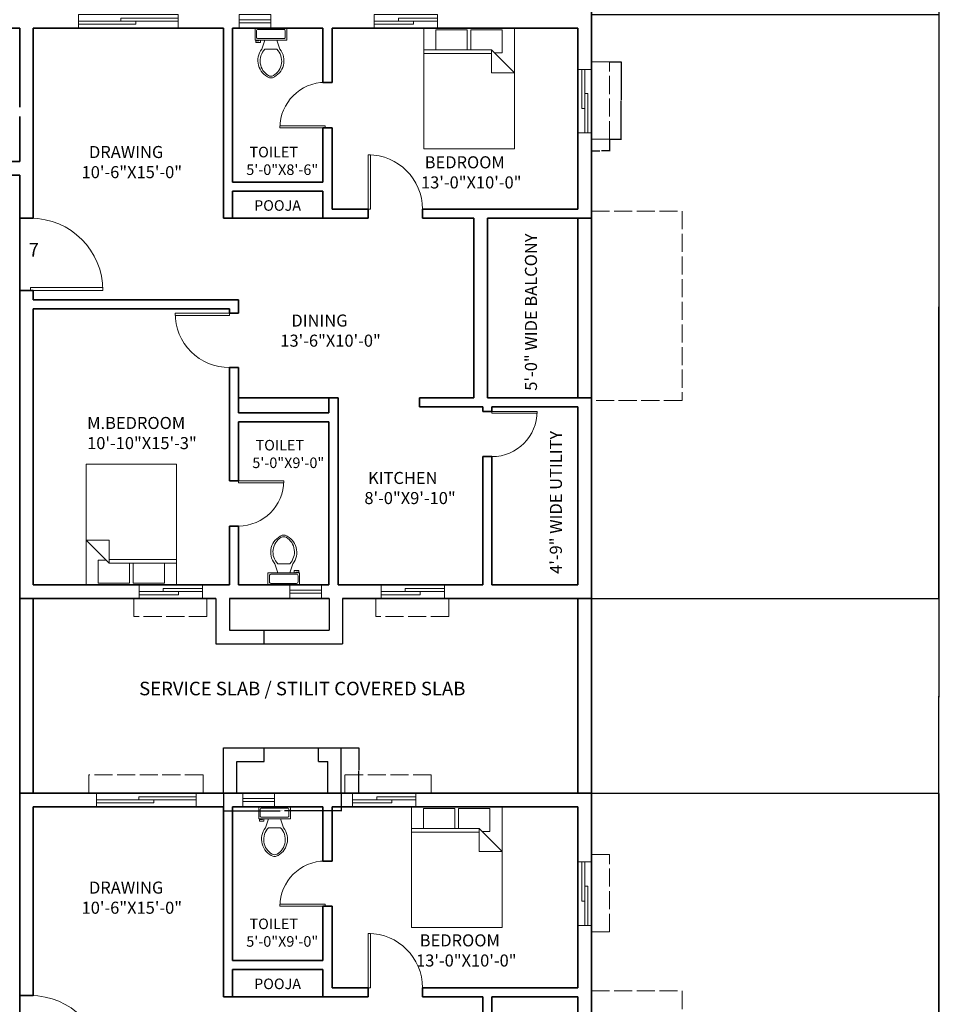
# Model space of a CAD drawing. Units: inches. Extents: x -69 to 2453, y 4803 to 7122.
# Tile 8 of 9: x 1843 to 2453, y 5759 to 6411. Entities that reach past the tile are written whole.
import ezdxf

# ---------------------------------------------------------------- set-up
doc = ezdxf.new("R2010")
doc.units = ezdxf.units.IN
doc.linetypes.add('ACAD_ISO02W100', pattern=[15, 12, -3])
for name, color, linetype, lineweight in [('A-ANNO-DIMS', 2, 'Continuous', 18), ('A-ANNO-IDEN', 2, 'Continuous', 18), ('A-AREA-IDEN', 7, 'Continuous', 18), ('A-DOOR', 3, 'Continuous', 18), ('A-FLOR-FIXT', 9, 'Continuous', 18), ('A-FLOR-OVHD', 8, 'ACAD_ISO02W100', 13), ('A-FURN', 8, 'Continuous', 18), ('A-GLAZ', 244, 'Continuous', 18), ('A-WALL', 7, 'Continuous', 35), ('A-WALL-SRVC', 7, 'Continuous', 30)]:
    doc.layers.add(name, color=color, linetype=linetype, lineweight=lineweight)
doc.styles.get("Standard").update_dxf_attribs({"font": 'arial.ttf'})
doc.dimstyles.get("Standard").update_dxf_attribs({"dimtxt": 0.18, "dimasz": 0.18, "dimexe": 0.18, "dimexo": 0.0625, "dimgap": 0.09, "dimtad": 0, "dimtih": 1, "dimtoh": 1, "dimdec": 4, "dimzin": 0, "dimdsep": 46, "dimtxsty": 'Standard', "dimcen": 0.09, "dimadec": 0, "dimazin": 0, "dimtfac": 1, "dimtdec": 4, "dimtofl": 0, "dimtmove": 0, "dimatfit": 3, "dimfxl": 1, "dimtolj": 1, "dimtzin": 0, "dimarcsym": 0})

# ---------------------------------------------------------------- blocks, each defined once
blk = doc.blocks.new('*U12')
for p, q in [((-40, 0), (-40, -6)), ((0, 0), (0, -6))]:
    blk.add_line(p, q)
blk.add_lwpolyline([(0, 0), (0, 40), (-1.75, 40), (-1.75, 0)], close=True)
blk.add_arc((0, 0), 40, 90, 180)
blk = doc.blocks.new('*U17')
for p, q in [((0, 0), (0, 6)), ((40, 0), (40, 6))]:
    blk.add_line(p, q)
blk.add_lwpolyline([(0, 0), (0, -40), (1.75, -40), (1.75, 0)], close=True)
blk.add_arc((0, 0), 40, 270, 0)
blk = doc.blocks.new('*U16')
for p, q in [((0, 0), (0, -6)), ((40, 0), (40, -6))]:
    blk.add_line(p, q)
blk.add_lwpolyline([(0, 0), (0, 40), (1.75, 40), (1.75, 0)], close=True)
blk.add_arc((0, 0), 40, 0, 90)
blk = doc.blocks.new('*U11')
for p, q in [((-40, 0), (-40, 6)), ((0, 0), (0, 6))]:
    blk.add_line(p, q)
blk.add_lwpolyline([(0, 0), (0, -40), (-1.75, -40), (-1.75, 0)], close=True)
blk.add_arc((0, 0), 40, 180, 270)
blk = doc.blocks.new('*U13')
for p, q in [((0, 0), (0, -6)), ((40, 0), (40, -6))]:
    blk.add_line(p, q)
blk.add_lwpolyline([(0, 0), (0, 40), (1.75, 40), (1.75, 0)], close=True)
blk.add_arc((0, 0), 40, 0, 90)
blk = doc.blocks.new('Bed - Queen')
for p, q in [((0, -80.00003), (0, 0)), ((0, 0), (59.99999, 0)), ((59.99999, 0), (59.99999, -80.00003)), ((7.99999, -1.2), (28.79998, -1.2)), ((7.99999, -14.4), (7.99999, -1.2)), ((28.79998, -1.2), (28.79998, -14.4)), ((31.19999, -1.2), (51.99999, -1.2)), ((31.19999, -14.4), (31.19999, -1.2)), ((51.99999, -1.2), (51.99999, -16.4)), ((0, -14.4), (44.8, -14.4)), ((44.8, -16.8), (0, -16.8)), ((59.99999, -29.6), (44.8, -14.4)), ((44.8, -14.4), (44.8, -29.6)), ((51.99999, -16.4), (46.79936, -16.4)), ((44.8, -29.6), (59.99999, -29.6)), ((59.99999, -80.00003), (0, -80.00003))]:
    blk.add_line(p, q)
blk = doc.blocks.new('*U33')
for p, q in [((9.5, -6), (9.5, -2)), ((-10, -8.5), (-8, -8.5)), ((-10, -9.5), (-10, -8.5)), ((-7, -9.5), (-10, -9.5)), ((-8, -8.5), (-8, -8)), ((-7, -8), (-7, -9.5)), ((-4, -8), (-6, -14)), ((4, -8), (6, -14)), ((4, -14), (-4, -14))]:
    blk.add_line(p, q)
blk.add_lwpolyline([(10.5, -8), (10.5, 0), (-10.5, 0), (-10.5, -8)], close=True)
for points in [[(-9.5, -2), (-9.5, -6)], [(8.5, -1), (-8.5, -1)], [(-8.5, -7), (8.5, -7)]]:
    blk.add_lwpolyline(points)
for centre, radius, start, end in [((-8.62, -1.88), 0.884, 81.8699, 188.1301), ((-8.62, -6.12), 0.884, 171.8699, 278.1301), ((8.62, -1.88), 0.884, 351.8699, 98.1301), ((8.62, -6.12), 0.884, 261.8699, 8.1301), ((3.52, -21.58), 12.17, 141.46911, 247.97143), ((4.2, -21.82), 11.33, 136.36773, 238.94682), ((-3.52, -21.58), 12.17, 292.02843, 38.53071), ((-4.2, -21.82), 11.33, 301.05301, 43.63209), ((0, -27.88), 4, 245.73182, 294.26817), ((0, -29), 4, 254.86053, 285.13947)]:
    blk.add_arc(centre, radius, start, end)
blk = doc.blocks.new('WINDOW-VENT-21IN')
for p, q in [((0, 5.5), (21, 5.5)), ((0, 3.5), (21, 3.5))]:
    blk.add_line(p, q)
blk.add_lwpolyline([(0, 9), (21, 9), (21, 0), (0, 0)], close=True)
blk = doc.blocks.new('WINDOW-SLIDING-42IN')
for p, q in [((2.5, 42), (2.5, 16)), ((4.5, 42), (4.5, 0)), ((4.5, 26), (6.5, 26)), ((6.5, 26), (6.5, 0)), ((4.5, 16), (2.5, 16))]:
    blk.add_line(p, q)
blk.add_lwpolyline([(0, 42), (9, 42), (9, 0), (0, 0)], close=True)
blk = doc.blocks.new('WINDOW-SLIDING-66IN')
for p, q in [((66, 4.5), (0, 4.5)), ((38, 2.5), (0, 2.5)), ((66, 6.5), (28, 6.5)), ((28, 4.5), (28, 6.5)), ((38, 4.5), (38, 2.5))]:
    blk.add_line(p, q)
blk.add_lwpolyline([(66, 9), (66, 0), (0, 0), (0, 9)], close=True)
blk = doc.blocks.new('SUNSHADE-48IN')
for p, q in [((0, 0), (0, 12)), ((48.4, 12), (48.4, 0)), ((48.4, 0), (0, 0))]:
    blk.add_line(p, q)
blk = doc.blocks.new('SUNSHADE-57IN')
for p, q in [((57.14, 12), (0, 12)), ((0, 12), (0, 0)), ((57.14, 0), (57.14, 12))]:
    blk.add_line(p, q)
blk = doc.blocks.new('SUNSHADE-51IN')
for p, q in [((12, 51.36), (0, 51.36)), ((12, 0), (12, 51.36)), ((0, 0), (12, 0))]:
    blk.add_line(p, q)
blk = doc.blocks.new('SUNSHADE-76IN')
for p, q in [((75.65, 12), (0, 12)), ((0, 12), (0, 0)), ((75.65, 0), (75.65, 12))]:
    blk.add_line(p, q)
blk = doc.blocks.new('SERVICE-BAY-78IN')
for p, q in [((0, 30), (78.14, 30)), ((0, 0), (0, 30)), ((27.07, 21), (27.07, 30)), ((63.07, 21), (63.07, 30)), ((78.14, 0), (78.14, 30)), ((9, 0), (9, 21)), ((9, 21), (27.07, 21)), ((63.07, 21), (69.14, 21)), ((69.14, 0), (69.14, 21))]:
    blk.add_line(p, q)
blk = doc.blocks.new('*D65')
at = {"layer": 'A-ANNO-DIMS', "color": 0, "lineweight": -2, "transparency": 16777216}
for p, q in [((2234.07, 6383.4), (2241.89, 6383.4)), ((2241.71, 6383.22), (2241.71, 6357.9)), ((2241.71, 6332.22), (2241.71, 6357.53)), ((2234.07, 6332.04), (2241.89, 6332.04))]:
    blk.add_line(p, q, dxfattribs=at)
at = {"layer": 'A-ANNO-DIMS', "color": 0, "transparency": 16777216}
for points in [[(2241.68, 6383.22), (2241.74, 6383.22), (2241.71, 6383.4)], [(2241.68, 6332.22), (2241.74, 6332.22), (2241.71, 6332.04)]]:
    blk.add_solid(points, dxfattribs=at)
at = {"layer": 'Defpoints', "color": 0, "transparency": 16777216}
for p in [(2234.01, 6383.4), (2241.71, 6383.4), (2234.01, 6332.04)]:
    blk.add_point(p, dxfattribs=at)
at = {"layer": 'A-ANNO-DIMS', "color": 0, "transparency": 16777216, "insert": (2241.71, 6357.72), "char_height": 0.18, "attachment_point": 5}
blk.add_mtext('\\A1;SUNSHADE 51 TYP.', dxfattribs=at)
blk = doc.blocks.new('*D66')
at = {"layer": 'A-ANNO-DIMS', "color": 0, "lineweight": -2, "transparency": 16777216}
for p, q in [((2222.01, 6331.97), (2222.01, 6324.15)), ((2234.01, 6331.97), (2234.01, 6324.15)), ((2222.19, 6324.33), (2227.49, 6324.33)), ((2233.83, 6324.33), (2228.53, 6324.33))]:
    blk.add_line(p, q, dxfattribs=at)
at = {"layer": 'A-ANNO-DIMS', "color": 0, "transparency": 16777216}
for points in [[(2222.19, 6324.36), (2222.19, 6324.3), (2222.01, 6324.33)], [(2233.83, 6324.36), (2233.83, 6324.3), (2234.01, 6324.33)]]:
    blk.add_solid(points, dxfattribs=at)
at = {"layer": 'Defpoints', "color": 0, "transparency": 16777216}
for p in [(2222.01, 6332.04), (2234.01, 6332.04), (2234.01, 6324.33)]:
    blk.add_point(p, dxfattribs=at)
at = {"layer": 'A-ANNO-DIMS', "color": 0, "transparency": 16777216, "insert": (2228.01, 6324.33), "char_height": 0.18, "attachment_point": 5}
blk.add_mtext('\\A1;12 TYP.', dxfattribs=at)
blk = doc.blocks.new('*D69')
at = {"layer": 'A-ANNO-DIMS', "color": 0, "lineweight": -2, "transparency": 16777216}
for p, q in [((1978.01, 5898.65), (1978.01, 5886.81)), ((2056.15, 5898.65), (2056.15, 5886.81)), ((1978.19, 5886.99), (2015.68, 5886.99)), ((2055.97, 5886.99), (2018.48, 5886.99))]:
    blk.add_line(p, q, dxfattribs=at)
at = {"layer": 'A-ANNO-DIMS', "color": 0, "transparency": 16777216}
for points in [[(1978.19, 5887.02), (1978.19, 5886.96), (1978.01, 5886.99)], [(2055.97, 5887.02), (2055.97, 5886.96), (2056.15, 5886.99)]]:
    blk.add_solid(points, dxfattribs=at)
at = {"layer": 'Defpoints', "color": 0, "transparency": 16777216}
for p in [(1978.01, 5898.72), (2056.15, 5898.72), (2056.15, 5886.99)]:
    blk.add_point(p, dxfattribs=at)
at = {"layer": 'A-ANNO-DIMS', "color": 0, "transparency": 16777216, "insert": (2017.08, 5886.99), "char_height": 0.18, "attachment_point": 5}
blk.add_mtext('\\A1;SERVICE BAY 78 TYP.', dxfattribs=at)
blk = doc.blocks.new('*D70')
at = {"layer": 'A-ANNO-DIMS', "color": 0, "lineweight": -2, "transparency": 16777216}
for p, q in [((2056.21, 5928.72), (2068.05, 5928.72)), ((2067.87, 5928.54), (2067.87, 5913.9)), ((2067.87, 5898.9), (2067.87, 5913.53)), ((2056.21, 5898.72), (2068.05, 5898.72))]:
    blk.add_line(p, q, dxfattribs=at)
at = {"layer": 'A-ANNO-DIMS', "color": 0, "transparency": 16777216}
for points in [[(2067.84, 5928.54), (2067.9, 5928.54), (2067.87, 5928.72)], [(2067.84, 5898.9), (2067.9, 5898.9), (2067.87, 5898.72)]]:
    blk.add_solid(points, dxfattribs=at)
at = {"layer": 'Defpoints', "color": 0, "transparency": 16777216}
for p in [(2056.15, 5928.72), (2067.87, 5928.72), (2056.15, 5898.72)]:
    blk.add_point(p, dxfattribs=at)
at = {"layer": 'A-ANNO-DIMS', "color": 0, "transparency": 16777216, "insert": (2067.87, 5913.72), "char_height": 0.18, "attachment_point": 5}
blk.add_mtext('\\A1;30 TYP.', dxfattribs=at)
blk = doc.blocks.new('*D90')
at = {"layer": 'A-ANNO-DIMS', "color": 0, "lineweight": -2, "transparency": 16777216}
for p, q in [((2222.07, 5898.72), (2452.44, 5898.72)), ((2452.26, 5898.54), (2452.26, 5705.4)), ((2452.26, 5511.9), (2452.26, 5705.03)), ((2222.07, 5511.72), (2452.44, 5511.72))]:
    blk.add_line(p, q, dxfattribs=at)
at = {"layer": 'A-ANNO-DIMS', "color": 0, "transparency": 16777216}
for points in [[(2452.23, 5898.54), (2452.29, 5898.54), (2452.26, 5898.72)], [(2452.23, 5511.9), (2452.29, 5511.9), (2452.26, 5511.72)]]:
    blk.add_solid(points, dxfattribs=at)
at = {"layer": 'Defpoints', "color": 0, "transparency": 16777216}
for p in [(2222.01, 5898.72), (2452.26, 5898.72), (2222.01, 5511.72)]:
    blk.add_point(p, dxfattribs=at)
at = {"layer": 'A-ANNO-DIMS', "color": 0, "transparency": 16777216, "insert": (2452.26, 5705.22), "char_height": 0.18, "attachment_point": 5}
blk.add_mtext('\\A1;387', dxfattribs=at)
blk = doc.blocks.new('*D91')
at = {"layer": 'A-ANNO-DIMS', "color": 0, "lineweight": -2, "transparency": 16777216}
for p, q in [((2222.07, 6027.72), (2452.44, 6027.72)), ((2452.26, 6027.54), (2452.26, 5963.4)), ((2452.26, 5898.9), (2452.26, 5963.03)), ((2222.07, 5898.72), (2452.44, 5898.72))]:
    blk.add_line(p, q, dxfattribs=at)
at = {"layer": 'A-ANNO-DIMS', "color": 0, "transparency": 16777216}
for points in [[(2452.23, 6027.54), (2452.29, 6027.54), (2452.26, 6027.72)], [(2452.23, 5898.9), (2452.29, 5898.9), (2452.26, 5898.72)]]:
    blk.add_solid(points, dxfattribs=at)
at = {"layer": 'Defpoints', "color": 0, "transparency": 16777216}
for p in [(2222.01, 6027.72), (2452.26, 6027.72), (2222.01, 5898.72)]:
    blk.add_point(p, dxfattribs=at)
at = {"layer": 'A-ANNO-DIMS', "color": 0, "transparency": 16777216, "insert": (2452.26, 5963.22), "char_height": 0.18, "attachment_point": 5}
blk.add_mtext('\\A1;129', dxfattribs=at)
blk = doc.blocks.new('*D92')
at = {"layer": 'A-ANNO-DIMS', "color": 0, "lineweight": -2, "transparency": 16777216}
for p, q in [((2222.07, 6414.72), (2452.44, 6414.72)), ((2452.26, 6414.54), (2452.26, 6221.4)), ((2452.26, 6027.9), (2452.26, 6221.03)), ((2222.07, 6027.72), (2452.44, 6027.72))]:
    blk.add_line(p, q, dxfattribs=at)
at = {"layer": 'A-ANNO-DIMS', "color": 0, "transparency": 16777216}
for points in [[(2452.23, 6414.54), (2452.29, 6414.54), (2452.26, 6414.72)], [(2452.23, 6027.9), (2452.29, 6027.9), (2452.26, 6027.72)]]:
    blk.add_solid(points, dxfattribs=at)
at = {"layer": 'Defpoints', "color": 0, "transparency": 16777216}
for p in [(2222.01, 6414.72), (2452.26, 6414.72), (2222.01, 6027.72)]:
    blk.add_point(p, dxfattribs=at)
at = {"layer": 'A-ANNO-DIMS', "color": 0, "transparency": 16777216, "insert": (2452.26, 6221.22), "char_height": 0.18, "attachment_point": 5}
blk.add_mtext('\\A1;387', dxfattribs=at)
blk = doc.blocks.new('*D96')
at = {"layer": 'A-ANNO-DIMS', "color": 0, "lineweight": -2, "transparency": 16777216}
for p, q in [((2044.63, 7006.72), (2452.44, 7006.72)), ((2452.26, 7006.54), (2452.26, 5962.4)), ((2452.26, 4917.9), (2452.26, 5962.03)), ((2143.12, 4917.72), (2452.44, 4917.72))]:
    blk.add_line(p, q, dxfattribs=at)
at = {"layer": 'A-ANNO-DIMS', "color": 0, "transparency": 16777216}
for points in [[(2452.23, 7006.54), (2452.29, 7006.54), (2452.26, 7006.72)], [(2452.23, 4917.9), (2452.29, 4917.9), (2452.26, 4917.72)]]:
    blk.add_solid(points, dxfattribs=at)
at = {"layer": 'Defpoints', "color": 0, "transparency": 16777216}
for p in [(2044.57, 7006.72), (2452.26, 7006.72), (2143.06, 4917.72)]:
    blk.add_point(p, dxfattribs=at)
at = {"layer": 'A-ANNO-DIMS', "color": 0, "transparency": 16777216, "insert": (2452.26, 5962.22), "char_height": 0.18, "attachment_point": 5}
blk.add_mtext('\\A1;2089', dxfattribs=at)

msp = doc.modelspace()

# ---------------------------------------------------------------- linework, layer by layer
at = {"layer": 'A-FLOR-OVHD'}
for p, q in [((2222.01, 6284.36), (2282.01, 6284.36)), ((2282.01, 6284.36), (2282.01, 6158.85)), ((2282.01, 6158.85), (2222.01, 6158.85)), ((2222.01, 5767.63), (2282.01, 5767.63)), ((2282.01, 5767.63), (2282.01, 5646.75))]:
    msp.add_line(p, q, dxfattribs=at)
at = {"layer": 'A-WALL'}
for p, q in [((2222.01, 6543.72), (2222.01, 5382.72)), ((1758.51, 6405.72), (1843.01, 6405.72)), ((1843.01, 6405.72), (1843.01, 6353.22)), ((1852.01, 6405.72), (1852.01, 6279.72)), ((1852.01, 6405.72), (1978.01, 6405.72)), ((1978.01, 6405.72), (1978.01, 6279.72)), ((1984.01, 6405.72), (1984.01, 6303.72)), ((1984.01, 6405.72), (2044.01, 6405.72)), ((2044.01, 6405.72), (2044.01, 6369.72)), ((2050.01, 6405.72), (2050.01, 6369.72)), ((2050.01, 6405.72), (2213.01, 6405.72)), ((2213.01, 6405.72), (2213.01, 6285.72)), ((2044.01, 6369.72), (2050.01, 6369.72)), ((1843.01, 6347.22), (1843.01, 6317.22)), ((2044.01, 6339.72), (2050.01, 6339.72)), ((2044.01, 6339.72), (2044.01, 6303.72)), ((2050.01, 6339.72), (2050.01, 6285.72)), ((1814.76, 6317.22), (1843.01, 6317.22)), ((1749.51, 6308.22), (1843.01, 6308.22)), ((1843.01, 6308.22), (1843.01, 5382.72)), ((1984.01, 6303.72), (2044.01, 6303.72)), ((1984.01, 6297.72), (2044.01, 6297.72)), ((1984.01, 6297.72), (1984.01, 6279.72)), ((2044.01, 6297.72), (2044.01, 6279.72)), ((2050.01, 6285.72), (2074.01, 6285.72)), ((2074.01, 6285.72), (2074.01, 6279.72)), ((2110.01, 6285.72), (2110.01, 6279.72)), ((2110.01, 6285.72), (2213.01, 6285.72)), ((1852.01, 6279.72), (1843.01, 6279.72)), ((1978.01, 6279.72), (2074.01, 6279.72)), ((2110.01, 6279.72), (2144.01, 6279.72)), ((2144.01, 6279.72), (2144.01, 6160.72)), ((2153.01, 6279.72), (2153.01, 6160.72)), ((2153.01, 6279.72), (2222.01, 6279.72)), ((2213.01, 6279.72), (2213.01, 6160.72)), ((1852.01, 6231.72), (1843.01, 6231.72)), ((1852.01, 6231.72), (1852.01, 6225.72)), ((1852.01, 6225.72), (1988.01, 6225.72)), ((1988.01, 6225.72), (1988.01, 6216.72)), ((1852.01, 6219.72), (1982.01, 6219.72)), ((1852.01, 6219.72), (1852.01, 6036.72)), ((1982.01, 6219.72), (1982.01, 6216.72)), ((1982.01, 6216.72), (1988.01, 6216.72)), ((1982.01, 6180.72), (1988.01, 6180.72)), ((1982.01, 6180.72), (1982.01, 6105.72)), ((1988.01, 6180.72), (1988.01, 6150.72)), ((1988.01, 6160.72), (2054.01, 6160.72)), ((2048.01, 6160.72), (2048.01, 6150.72)), ((2054.01, 6160.72), (2054.01, 6036.72)), ((2108.01, 6160.72), (2108.01, 6154.72)), ((2108.01, 6160.72), (2144.01, 6160.72)), ((2153.01, 6160.72), (2222.01, 6160.72)), ((2150.01, 6154.72), (2108.01, 6154.72)), ((2150.01, 6154.72), (2150.01, 6151.72)), ((2156.01, 6154.72), (2156.01, 6151.72)), ((2156.01, 6154.72), (2213.01, 6154.72)), ((2213.01, 6154.72), (2213.01, 6036.72)), ((1988.01, 6150.72), (2048.01, 6150.72)), ((2150.01, 6151.72), (2156.01, 6151.72)), ((1988.01, 6144.72), (2048.01, 6144.72)), ((1988.01, 6144.72), (1988.01, 6105.72)), ((2048.01, 6144.72), (2048.01, 6036.72)), ((2150.01, 6121.72), (2156.01, 6121.72)), ((2150.01, 6121.72), (2150.01, 6036.72)), ((2156.01, 6121.72), (2156.01, 6036.72)), ((1988.01, 6105.72), (1982.01, 6105.72)), ((1988.01, 6075.72), (1982.01, 6075.72)), ((1982.01, 6075.72), (1982.01, 6036.72)), ((1988.01, 6075.72), (1988.01, 6036.72)), ((1852.01, 6036.72), (1982.01, 6036.72)), ((1988.01, 6036.72), (2048.01, 6036.72)), ((2054.01, 6036.72), (2150.01, 6036.72)), ((2156.01, 6036.72), (2213.01, 6036.72)), ((1843.01, 6027.72), (1973.01, 6027.72)), ((1852.01, 6027.72), (1852.01, 5898.72)), ((1982.01, 6027.72), (2048.06, 6027.72)), ((2057.06, 6027.72), (2222.01, 6027.72)), ((2213.01, 6027.72), (2213.01, 5898.72)), ((1843.01, 5898.72), (2222.01, 5898.72)), ((1852.01, 5889.72), (1978.01, 5889.72)), ((1852.01, 5889.72), (1852.01, 5764.52)), ((1978.01, 5889.72), (1978.01, 5763.72)), ((1984.01, 5889.72), (1984.01, 5787.72)), ((1984.01, 5889.72), (2044.01, 5889.72)), ((2044.01, 5889.72), (2044.01, 5853.72)), ((2050.01, 5889.72), (2050.01, 5853.72)), ((2050.01, 5889.72), (2213.01, 5889.72)), ((2213.01, 5889.72), (2213.01, 5769.72)), ((2044.01, 5853.72), (2050.01, 5853.72)), ((2044.01, 5823.72), (2050.01, 5823.72)), ((2044.01, 5823.72), (2044.01, 5787.72)), ((2050.01, 5823.72), (2050.01, 5769.72)), ((1984.01, 5787.72), (2044.01, 5787.72)), ((1984.01, 5781.72), (2044.01, 5781.72)), ((1984.01, 5781.72), (1984.01, 5763.72)), ((2044.01, 5781.72), (2044.01, 5763.72)), ((2050.01, 5769.72), (2074.01, 5769.72)), ((2074.01, 5769.72), (2074.01, 5763.72)), ((2110.01, 5769.72), (2110.01, 5763.72)), ((2110.01, 5769.72), (2213.01, 5769.72)), ((1852.01, 5764.52), (1843.01, 5764.52)), ((1978.01, 5763.72), (2074.01, 5763.72)), ((2110.01, 5763.72), (2150.01, 5763.72)), ((2150.01, 5763.72), (2150.01, 5648.72)), ((2156.01, 5763.72), (2156.01, 5648.72)), ((2156.01, 5763.72), (2213.01, 5763.72)), ((2213.01, 5763.72), (2213.01, 5648.72))]:
    msp.add_line(p, q, dxfattribs=at)
at = {"layer": 'A-WALL-SRVC'}
for p, q in [((1973.01, 6027.72), (1973.01, 5997.72)), ((1982.01, 6027.72), (1982.01, 6006.72)), ((2048.06, 6027.72), (2048.06, 6006.72)), ((2057.06, 6027.72), (2057.06, 5997.72)), ((1982.01, 6006.72), (2048.06, 6006.72)), ((2004.83, 6006.72), (2004.83, 5997.72)), ((1973.01, 5997.72), (2057.06, 5997.72))]:
    msp.add_line(p, q, dxfattribs=at)

# ---------------------------------------------------------------- block references
at = {"layer": 'A-DOOR'}
for name, p, xscale, yscale, zscale, rotation in [('*U11', (2045.51, 6339.72), 0.75, 0.75, 0.75, 270.0000000000001), ('*U12', (1850.21, 6231.72), 1.199999999999977, 1.199999999999977, 1.199999999999977, 270.0000000000001), ('*U17', (1982.01, 6216.72), 0.9, 0.9, 0.9, 270), ('*U13', (2156.01, 6151.72), 0.75, 0.75, 0.75, 270.0000000000001), ('*U13', (1988.01, 6105.72), 0.75, 0.75, 0.75, 270.0000000000001), ('*U11', (2045.51, 5823.72), 0.75, 0.75, 0.75, 270.0000000000001), ('*U12', (1850.21, 5716.52), 1.199999999999977, 1.199999999999977, 1.199999999999977, 270.0000000000001)]:
    msp.add_blockref(name, p, dxfattribs=dict(at, xscale=xscale, yscale=yscale, zscale=zscale, rotation=rotation))
at = {"layer": 'A-DOOR', "xscale": 0.9, "yscale": 0.9, "zscale": 0.9}
for p in [(2074.01, 6285.72), (2074.01, 5769.72)]:
    msp.add_blockref('*U16', p, dxfattribs=at)
at = {"layer": 'A-FLOR-FIXT'}
for p in [(2009.52, 6405.72), (2011.93, 5889.72)]:
    msp.add_blockref('*U33', p, dxfattribs=at)
at = {"layer": 'A-FLOR-FIXT', "rotation": 180}
msp.add_blockref('*U33', (2018.01, 6036.72), dxfattribs=at)
at = {"layer": 'A-FLOR-OVHD'}
for name, p in [('SUNSHADE-51IN', (2222.01, 6332.04)), ('SUNSHADE-48IN', (1918.74, 6015.72)), ('SUNSHADE-48IN', (2079.05, 6015.72)), ('SUNSHADE-76IN', (1888.88, 5898.72)), ('SUNSHADE-57IN', (2058.57, 5898.72)), ('SUNSHADE-51IN', (2222.01, 5806.72))]:
    msp.add_blockref(name, p, dxfattribs=at)
at = {"layer": 'A-FURN'}
for p in [(2110.87, 6405.72), (2102.71, 5889.72)]:
    msp.add_blockref('Bed - Queen', p, dxfattribs=at)
at = {"layer": 'A-FURN', "rotation": 180}
msp.add_blockref('Bed - Queen', (1947.01, 6036.72), dxfattribs=at)
at = {"layer": 'A-GLAZ'}
for name, p in [('WINDOW-SLIDING-66IN', (1882.01, 6405.72)), ('WINDOW-VENT-21IN', (1988.52, 6405.72)), ('WINDOW-SLIDING-42IN', (2213.01, 6336.37)), ('WINDOW-VENT-21IN', (2021.99, 6027.72)), ('WINDOW-SLIDING-66IN', (1893.95, 5889.72)), ('WINDOW-VENT-21IN', (1990.93, 5889.72)), ('WINDOW-SLIDING-42IN', (2213.01, 5811.06))]:
    msp.add_blockref(name, p, dxfattribs=at)
for p, rotation in [((2078.01, 6414.72), 270.0000000000009), ((1922.19, 6036.72), 269.9999999999988), ((2082.5, 6036.72), 270.0000000000009), ((2063.66, 5898.72), 269.9999999999984)]:
    msp.add_blockref('WINDOW-SLIDING-42IN', p, dxfattribs=dict(at, rotation=rotation))
at = {"layer": 'A-WALL-SRVC'}
msp.add_blockref('SERVICE-BAY-78IN', (1978.01, 5898.72), dxfattribs=at)

# ---------------------------------------------------------------- texts
at = {"layer": 'A-ANNO-IDEN', "insert": (1848.93, 6263.27), "char_height": 8, "attachment_point": 1}
msp.add_mtext_dynamic_manual_height_columns('{\\H1.125x;7} ', width=10.4994, gutter_width=12.5, heights=[0], dxfattribs=at)
at = {"layer": 'A-AREA-IDEN', "attachment_point": 1}
for s, width, insert, char_height in [('  DRAWING\\P10\'-6"X15\'-0"', 66.0939, (1884.05, 6327.59), 8), (' TOILET\\P5\'-0"X8\'-6"', 45.2002, (1993.2, 6327.06), 7), (' BEDROOM\\P13\'-0"X10\'-0"', 64.9911, (2109.01, 6320.78), 8), ('POOJA', 33.9191, (1998.36, 6291.65), 7), ('   DINING\\P13\'-6"X10\'-0"', 63.2359, (2015.77, 6215.9), 8), ('M.BEDROOM\\P10\'-10"X15\'-3"', 69.6032, (1887.72, 6148.02), 8), (' TOILET\\P5\'-0"X9\'-0"', 45.2002, (1997.2, 6132.8), 7), (' KITCHEN\\P8\'-0"X9\'-10"', 58.1282, (2071.46, 6111.59), 8), ('SERVICE SLAB / STILIT COVERED SLAB', 244.2019, (1922.18, 5972.53), 9), ('  DRAWING\\P10\'-6"X15\'-0"', 66.0939, (1884.05, 5840.09), 8), (' TOILET\\P5\'-0"X9\'-0"', 45.2002, (1993.2, 5815.57), 7), (' BEDROOM\\P13\'-0"X10\'-0"', 64.9911, (2105.73, 5805.11), 8), ('POOJA', 33.9191, (1998.36, 5775.79), 7)]:
    msp.add_mtext_dynamic_manual_height_columns(s, width=width, gutter_width=12.5, heights=[0], dxfattribs=dict(at, insert=insert, char_height=char_height))
at = {"layer": 'A-AREA-IDEN', "char_height": 8, "attachment_point": 1, "rotation": 90}
for s, width, insert in [('5\'-0" WIDE BALCONY', 114.3745, (2177.88, 6165.4)), ('4\'-9" WIDE UTILITY', 99.5525, (2194.4, 6044.01))]:
    msp.add_mtext_dynamic_manual_height_columns(s, width=width, gutter_width=12.5, heights=[0], dxfattribs=dict(at, insert=insert))

# ---------------------------------------------------------------- dimensions: what is measured, and where the dimension line sits
at = {"layer": 'A-ANNO-DIMS'}
for base, p1, p2, picture, middle in [((2452.26, 7006.72), (2143.06, 4917.72), (2044.57, 7006.72), '*D96', (2452.26, 5962.22)), ((2452.26, 6414.72), (2222.01, 6027.72), (2222.01, 6414.72), '*D92', (2452.26, 6221.22)), ((2452.26, 6027.72), (2222.01, 5898.72), (2222.01, 6027.72), '*D91', (2452.26, 5963.22)), ((2452.26, 5898.72), (2222.01, 5511.72), (2222.01, 5898.72), '*D90', (2452.26, 5705.22))]:
    dim = msp.add_linear_dim(base=base, p1=p1, p2=p2, angle=90, dimstyle='Standard', override={"dimdec": 0, "dimlfac": 1, "dimrnd": 0, "dimzin": 0, "dimdsep": 46, "dimlunit": 2}, dxfattribs=at)
    dim.commit()
    dim.dimension.update_dxf_attribs({"geometry": picture, "text_midpoint": middle})
for base, p1, p2, text, picture, middle in [((2241.71, 6383.4), (2234.01, 6332.04), (2234.01, 6383.4), 'SUNSHADE <> TYP.', '*D65', (2241.71, 6357.72)), ((2067.87, 5928.72), (2056.15, 5898.72), (2056.15, 5928.72), '<> TYP.', '*D70', (2067.87, 5913.72))]:
    dim = msp.add_linear_dim(base=base, p1=p1, p2=p2, angle=90, text=text, dimstyle='Standard', override={"dimdec": 0, "dimlfac": 1, "dimrnd": 0, "dimzin": 0, "dimdsep": 46, "dimlunit": 2}, dxfattribs=at)
    dim.commit()
    dim.dimension.update_dxf_attribs({"geometry": picture, "text_midpoint": middle})
for base, p1, p2, text, picture, middle in [((2234.01, 6324.33), (2222.01, 6332.04), (2234.01, 6332.04), '<> TYP.', '*D66', (2228.01, 6324.33)), ((2056.15, 5886.99), (1978.01, 5898.72), (2056.15, 5898.72), 'SERVICE BAY <> TYP.', '*D69', (2017.08, 5886.99))]:
    dim = msp.add_linear_dim(base=base, p1=p1, p2=p2, text=text, dimstyle='Standard', override={"dimdec": 0, "dimlfac": 1, "dimrnd": 0, "dimzin": 0, "dimdsep": 46, "dimlunit": 2}, dxfattribs=at)
    dim.commit()
    dim.dimension.update_dxf_attribs({"geometry": picture, "text_midpoint": middle})

doc.saveas('drawing.dxf')
